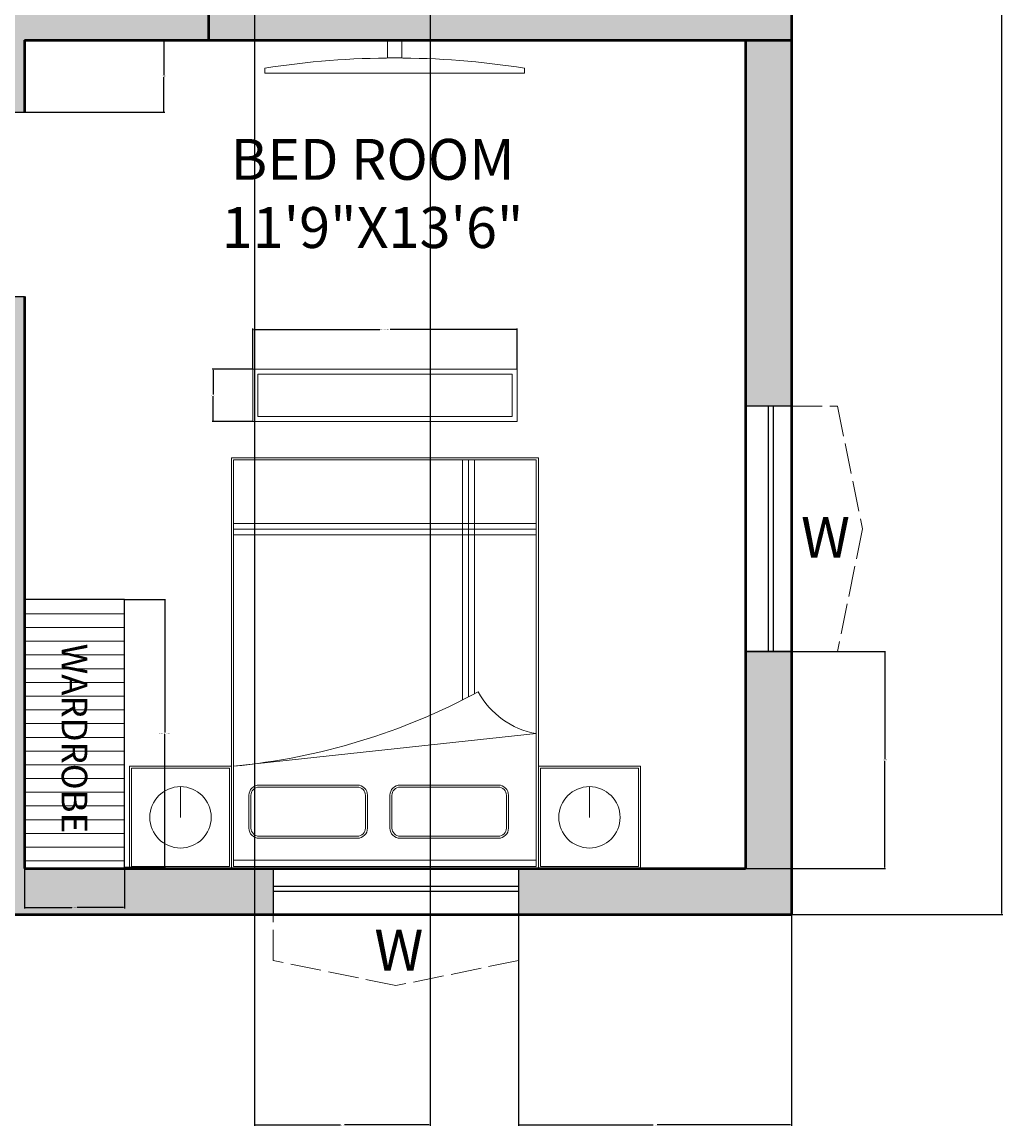
# Model space of a CAD drawing. Units: inches. Extents: x -75 to 416, y -487 to 70.
# Tile 3 of 5: x 224 to 416, y -487 to -271. Entities that reach past the tile are written whole.
import ezdxf

# ---------------------------------------------------------------- set-up
doc = ezdxf.new("R2010")
doc.units = ezdxf.units.IN
doc.header["$MEASUREMENT"] = 0
doc.linetypes.add('ACAD_ISO02W100', pattern=[15, 12, -3])
for name, color, linetype, lineweight in [('A-ANNO-DIMS', 2, 'Continuous', 18), ('A-ANNO-TEXT', 7, 'Continuous', 18), ('A-AREA-IDEN', 7, 'Continuous', 25), ('A-DOOR', 3, 'Continuous', 25), ('A-EQPM', 8, 'Continuous', 18), ('A-FLOR-CASE', 8, 'Continuous', 25), ('A-FLOR-CASE-PATT', 252, 'Continuous', 13), ('A-FURN', 8, 'Continuous', 18), ('A-GLAZ', 4, 'Continuous', 25), ('A-GLAZ-OVHD', 4, 'ACAD_ISO02W100', 13), ('A-WALL', 7, 'Continuous', 50), ('A-WALL-PATT', 252, 'Continuous', 13)]:
    doc.layers.add(name, color=color, linetype=linetype, lineweight=lineweight)
doc.styles.get("Standard").update_dxf_attribs({"font": 'arial.ttf'})
doc.dimstyles.get("Standard").update_dxf_attribs({"dimtxt": 0.18, "dimasz": 0.18, "dimexe": 0.18, "dimexo": 0.0625, "dimgap": 0.09, "dimtad": 0, "dimtih": 1, "dimtoh": 1, "dimdec": 4, "dimzin": 0, "dimdsep": 46, "dimtxsty": 'Standard', "dimcen": 0.09, "dimadec": 0, "dimazin": 0, "dimtfac": 1, "dimtdec": 4, "dimtofl": 0, "dimtmove": 0, "dimatfit": 3, "dimfxl": 1, "dimtolj": 1, "dimtzin": 0, "dimarcsym": 0})

# ---------------------------------------------------------------- blocks, each defined once
blk = doc.blocks.new('A$C0EA4476A')
at = {"linetype": 'ByBlock', "lineweight": -2}
for p, q in [((0, 2.008), (0, 1.508)), ((0.5, 2.008), (0, 2.008)), ((0.01, 1.998), (0.01, 1.518)), ((0.49, 1.998), (0.01, 1.998)), ((0.49, 1.518), (0.49, 1.998)), ((0.5, 2.008), (2, 2.008)), ((0.5, 0), (0.5, 2.008)), ((0.5, 1.508), (0.5, 2.008)), ((0.51, 1.998), (1.99, 1.998)), ((0.51, 0.01), (0.51, 1.998)), ((1.99, 1.998), (1.99, 0.01)), ((2, 2.008), (2, 0)), ((2, 2.008), (2.5, 2.008)), ((2, 1.508), (2, 2.008)), ((2.01, 1.998), (2.49, 1.998)), ((2.01, 1.518), (2.01, 1.998)), ((2.49, 1.998), (2.49, 1.518)), ((2.5, 2.008), (2.5, 1.508)), ((0.51, 1.968), (1.99, 1.968)), ((0.696, 1.8603), (1.176, 1.8603)), ((0.696, 1.8503), (1.176, 1.8503)), ((1.3855, 1.8603), (1.8655, 1.8603)), ((1.3855, 1.8503), (1.8655, 1.8503)), ((0.646, 1.6503), (0.646, 1.8103)), ((0.656, 1.6503), (0.656, 1.8103)), ((1.216, 1.8103), (1.216, 1.6503)), ((1.226, 1.8103), (1.226, 1.6503)), ((1.3355, 1.6503), (1.3355, 1.8103)), ((1.3455, 1.6503), (1.3455, 1.8103)), ((1.9055, 1.8103), (1.9055, 1.6503)), ((1.9155, 1.8103), (1.9155, 1.6503)), ((0.25, 1.758), (0.25, 1.608)), ((2.25, 1.758), (2.25, 1.608)), ((1.176, 1.6103), (0.696, 1.6103)), ((1.176, 1.6003), (0.696, 1.6003)), ((1.8655, 1.6103), (1.3855, 1.6103)), ((1.8655, 1.6003), (1.3855, 1.6003)), ((0.01, 1.518), (0.49, 1.518)), ((2.49, 1.518), (2.01, 1.518)), ((0, 1.508), (0.5, 1.508)), ((1.99, 1.508), (0.51, 1.3488)), ((2.5, 1.508), (2, 1.508)), ((0.8115, 1.1534), (0.8115, 0.01)), ((0.8415, 1.1692), (0.8415, 0.01)), ((0.8715, 1.1845), (0.8715, 0.01)), ((0.51, 0.3775), (1.99, 0.3775)), ((0.51, 0.3495), (1.99, 0.3495)), ((0.51, 0.3216), (1.99, 0.3216)), ((1.99, 0.01), (0.51, 0.01)), ((2, 0), (0.5, 0))]:
    blk.add_line(p, q, dxfattribs=at)
for centre in [(0.25, 1.758), (2.25, 1.758)]:
    blk.add_circle(centre, 0.15, dxfattribs=at)
for centre, radius, start, end in [((0.696, 1.8103), 0.05, 90, 180), ((0.696, 1.8103), 0.04, 90, 180), ((1.176, 1.8103), 0.05, 0, 90), ((1.176, 1.8103), 0.04, 0, 90), ((1.3855, 1.8103), 0.05, 90, 180), ((1.3855, 1.8103), 0.04, 90, 180), ((1.8655, 1.8103), 0.05, 0, 90), ((1.8655, 1.8103), 0.04, 0, 90), ((0.696, 1.6503), 0.05, 180, 270), ((0.696, 1.6503), 0.04, 180, 270), ((1.176, 1.6503), 0.04, 270, 0), ((1.176, 1.6503), 0.05, 270, 0), ((1.3855, 1.6503), 0.05, 180, 270), ((1.3855, 1.6503), 0.04, 180, 270), ((1.8655, 1.6503), 0.05, 270, 0), ((1.8655, 1.6503), 0.04, 270, 0), ((2.2933, -1.6357), 3.1583, 95.5104, 118.3399), ((0.4397, 0.9519), 0.4031, 28.4688, 79.9557)]:
    blk.add_arc(centre, radius, start, end, dxfattribs=at)
blk = doc.blocks.new('A$C1A706E3E')
blk.add_blockref('A$C0EA4476A', (0, 0))
blk = doc.blocks.new('WIN-48IN')
for p, q in [((0, 9), (0, 0)), ((48, 9), (48, 0)), ((48, 5.5), (0, 5.5)), ((48, 4.5), (0, 4.5))]:
    blk.add_line(p, q)
blk = doc.blocks.new('WIN-SHADE-48IN')
at = {"ltscale": 0.5}
for p, q in [((0, 4.91), (0, 13.91)), ((48, 13.91), (48, 4.91)), ((24, 0), (0, 4.91)), ((48, 4.91), (24, 0))]:
    blk.add_line(p, q, dxfattribs=at)
blk = doc.blocks.new('DOOR-36IN')
for p, q in [((0, 9), (0, 0)), ((36, 9), (36, 0)), ((36, 4.5), (0, 4.5))]:
    blk.add_line(p, q)
blk = doc.blocks.new('TV-WALL-MOUNT')
for p, q in [((24, 6.49), (0, 6.49)), ((0, 6.49), (0, 5.49)), ((26.81, 6.49), (24, 6.49)), ((26.81, 6.49), (50.81, 6.49)), ((50.81, 6.49), (50.81, 5.49)), ((24, 3.49), (24, 0)), ((26.81, 3.49), (24, 3.49)), ((26.81, 3.49), (26.81, 0))]:
    blk.add_line(p, q)
blk.add_arc((25.41, 165.85), 162.36, 260.9976, 279.0024)
blk = doc.blocks.new('BENCH-BED-END')
for points in [[(0, 10.24), (51.71, 10.24), (51.71, 0), (0, 0)], [(1, 9.24), (50.71, 9.24), (50.71, 1), (1, 1)]]:
    blk.add_lwpolyline(points, close=True)
blk = doc.blocks.new('WARDROBE-OUTLINE')
for p, q in [((0, 52.38), (0, 0)), ((0, 0), (19.56, 0))]:
    blk.add_line(p, q)
blk = doc.blocks.new('*D24')
at = {"layer": 'A-ANNO-DIMS', "color": 0, "lineweight": -2, "transparency": 16777216}
for p, q in [((269.2, -338.66), (269.2, -330.79)), ((269.38, -330.97), (294.05, -330.97)), ((320.73, -330.97), (296.05, -330.97)), ((320.91, -338.66), (320.91, -330.79))]:
    blk.add_line(p, q, dxfattribs=at)
at = {"layer": 'A-ANNO-DIMS', "color": 0, "transparency": 16777216}
for points in [[(269.38, -330.94), (269.38, -331), (269.2, -330.97)], [(320.73, -330.94), (320.73, -331), (320.91, -330.97)]]:
    blk.add_solid(points, dxfattribs=at)
at = {"layer": 'Defpoints', "color": 0, "transparency": 16777216}
for p in [(320.91, -330.97), (269.2, -338.72), (320.91, -338.72)]:
    blk.add_point(p, dxfattribs=at)
at = {"layer": 'A-ANNO-DIMS', "color": 0, "transparency": 16777216, "insert": (295.05, -330.97), "char_height": 0.18, "attachment_point": 5}
blk.add_mtext('\\A1;BENCH 52 TYP.', dxfattribs=at)
blk = doc.blocks.new('*D25')
at = {"layer": 'A-ANNO-DIMS', "color": 0, "lineweight": -2, "transparency": 16777216}
for p, q in [((269.14, -338.72), (261.26, -338.72)), ((261.44, -338.9), (261.44, -343.66)), ((261.44, -348.78), (261.44, -344.02)), ((269.14, -348.96), (261.26, -348.96))]:
    blk.add_line(p, q, dxfattribs=at)
at = {"layer": 'A-ANNO-DIMS', "color": 0, "transparency": 16777216}
for points in [[(261.41, -338.9), (261.47, -338.9), (261.44, -338.72)], [(261.41, -348.78), (261.47, -348.78), (261.44, -348.96)]]:
    blk.add_solid(points, dxfattribs=at)
at = {"layer": 'Defpoints', "color": 0, "transparency": 16777216}
for p in [(261.44, -338.72), (269.2, -338.72), (269.2, -348.96)]:
    blk.add_point(p, dxfattribs=at)
at = {"layer": 'A-ANNO-DIMS', "color": 0, "transparency": 16777216, "insert": (261.44, -343.84), "char_height": 0.18, "attachment_point": 5}
blk.add_mtext('\\A1;10 TYP.', dxfattribs=at)
blk = doc.blocks.new('*D26')
at = {"layer": 'A-ANNO-DIMS', "color": 0, "lineweight": -2, "transparency": 16777216}
for p, q in [((244.17, -383.76), (252.15, -383.76)), ((251.97, -383.94), (251.97, -409.76)), ((251.97, -435.96), (251.97, -410.13)), ((244.17, -436.14), (252.15, -436.14))]:
    blk.add_line(p, q, dxfattribs=at)
at = {"layer": 'A-ANNO-DIMS', "color": 0, "transparency": 16777216}
for points in [[(251.94, -383.94), (252, -383.94), (251.97, -383.76)], [(251.94, -435.96), (252, -435.96), (251.97, -436.14)]]:
    blk.add_solid(points, dxfattribs=at)
at = {"layer": 'Defpoints', "color": 0, "transparency": 16777216}
for p in [(244.11, -383.76), (244.11, -436.14), (251.97, -436.14)]:
    blk.add_point(p, dxfattribs=at)
at = {"layer": 'A-ANNO-DIMS', "color": 0, "transparency": 16777216, "insert": (251.97, -409.95), "char_height": 0.18, "attachment_point": 5}
blk.add_mtext('\\A1;WARDROBE 52 TYP.', dxfattribs=at)
blk = doc.blocks.new('*D27')
at = {"layer": 'A-ANNO-DIMS', "color": 0, "lineweight": -2, "transparency": 16777216}
for p, q in [((224.55, -436.2), (224.55, -444.17)), ((244.11, -436.2), (244.11, -444.17)), ((224.73, -443.99), (233.8, -443.99)), ((243.93, -443.99), (234.86, -443.99))]:
    blk.add_line(p, q, dxfattribs=at)
at = {"layer": 'A-ANNO-DIMS', "color": 0, "transparency": 16777216}
for points in [[(224.73, -443.96), (224.73, -444.02), (224.55, -443.99)], [(243.93, -443.96), (243.93, -444.02), (244.11, -443.99)]]:
    blk.add_solid(points, dxfattribs=at)
at = {"layer": 'Defpoints', "color": 0, "transparency": 16777216}
for p in [(224.55, -436.14), (244.11, -436.14), (224.55, -443.99)]:
    blk.add_point(p, dxfattribs=at)
at = {"layer": 'A-ANNO-DIMS', "color": 0, "transparency": 16777216, "insert": (234.33, -443.99), "char_height": 0.18, "attachment_point": 5}
blk.add_mtext('\\A1;20 TYP.', dxfattribs=at)
blk = doc.blocks.new('*D35')
at = {"layer": 'A-ANNO-DIMS', "color": 0, "lineweight": -2, "transparency": 16777216}
for p, q in [((374.615553, 28.625508), (415.902741, 28.625508)), ((415.722741, 28.445508), (415.722741, -208.194492)), ((415.722741, -445.194492), (415.722741, -208.554492)), ((374.615553, -445.374492), (415.902741, -445.374492))]:
    blk.add_line(p, q, dxfattribs=at)
at = {"layer": 'A-ANNO-DIMS', "color": 0, "transparency": 16777216}
for points in [[(415.692741, 28.445508), (415.752741, 28.445508), (415.722741, 28.625508)], [(415.692741, -445.194492), (415.752741, -445.194492), (415.722741, -445.374492)]]:
    blk.add_solid(points, dxfattribs=at)
at = {"layer": 'Defpoints', "color": 0, "transparency": 16777216}
for p in [(374.553053, 28.625508), (374.553053, -445.374492), (415.722741, -445.374492)]:
    blk.add_point(p, dxfattribs=at)
at = {"layer": 'A-ANNO-DIMS', "color": 0, "transparency": 16777216, "insert": (415.722741, -208.374492), "char_height": 0.18, "attachment_point": 5}
blk.add_mtext('\\A1;474', dxfattribs=at)
blk = doc.blocks.new('*D42')
at = {"layer": 'A-ANNO-DIMS', "color": 0, "lineweight": -2, "transparency": 16777216}
for p, q in [((365.62, -393.93), (392.99, -393.93)), ((392.81, -394.11), (392.81, -414.97)), ((392.81, -436.19), (392.81, -415.33)), ((365.62, -436.37), (392.99, -436.37))]:
    blk.add_line(p, q, dxfattribs=at)
at = {"layer": 'A-ANNO-DIMS', "color": 0, "transparency": 16777216}
for points in [[(392.78, -394.11), (392.84, -394.11), (392.81, -393.93)], [(392.78, -436.19), (392.84, -436.19), (392.81, -436.37)]]:
    blk.add_solid(points, dxfattribs=at)
at = {"layer": 'Defpoints', "color": 0, "transparency": 16777216}
for p in [(365.55, -393.93), (365.55, -436.37), (392.81, -436.37)]:
    blk.add_point(p, dxfattribs=at)
at = {"layer": 'A-ANNO-DIMS', "color": 0, "transparency": 16777216, "insert": (392.81, -415.15), "char_height": 0.18, "attachment_point": 5}
blk.add_mtext('\\A1;42.444', dxfattribs=at)
blk = doc.blocks.new('*D51')
at = {"layer": 'A-ANNO-DIMS', "color": 0, "lineweight": -2, "transparency": 16777216}
for p, q in [((321.2, -445.44), (321.2, -486.72)), ((374.55, -445.44), (374.55, -486.72)), ((321.38, -486.54), (347.48, -486.54)), ((374.37, -486.54), (348.27, -486.54))]:
    blk.add_line(p, q, dxfattribs=at)
at = {"layer": 'A-ANNO-DIMS', "color": 0, "transparency": 16777216}
for points in [[(321.38, -486.51), (321.38, -486.57), (321.2, -486.54)], [(374.37, -486.51), (374.37, -486.57), (374.55, -486.54)]]:
    blk.add_solid(points, dxfattribs=at)
at = {"layer": 'Defpoints', "color": 0, "transparency": 16777216}
for p in [(321.2, -445.37), (374.55, -445.37), (321.2, -486.54)]:
    blk.add_point(p, dxfattribs=at)
at = {"layer": 'A-ANNO-DIMS', "color": 0, "transparency": 16777216, "insert": (347.88, -486.54), "char_height": 0.18, "attachment_point": 5}
blk.add_mtext('\\A1;53.35', dxfattribs=at)
blk = doc.blocks.new('*D56')
at = {"layer": 'A-ANNO-DIMS', "color": 0, "lineweight": -2, "transparency": 16777216}
for p, q in [((224.62, -274.37), (251.99, -274.37)), ((251.81, -274.55), (251.81, -281.25)), ((251.81, -288.31), (251.81, -281.61)), ((224.62, -288.49), (251.99, -288.49))]:
    blk.add_line(p, q, dxfattribs=at)
at = {"layer": 'A-ANNO-DIMS', "color": 0, "transparency": 16777216}
for points in [[(251.78, -274.55), (251.84, -274.55), (251.81, -274.37)], [(251.78, -288.31), (251.84, -288.31), (251.81, -288.49)]]:
    blk.add_solid(points, dxfattribs=at)
at = {"layer": 'Defpoints', "color": 0, "transparency": 16777216}
for p in [(224.55, -274.37), (224.55, -288.49), (251.81, -288.49)]:
    blk.add_point(p, dxfattribs=at)
at = {"layer": 'A-ANNO-DIMS', "color": 0, "transparency": 16777216, "insert": (251.81, -281.43), "char_height": 0.18, "attachment_point": 5}
blk.add_mtext('\\A1;14.116', dxfattribs=at)
blk = doc.blocks.new('*D71')
at = {"layer": 'A-ANNO-DIMS', "color": 0, "lineweight": -2, "transparency": 16777216}
for p, q in [((303.87, -261.95), (303.87, -486.72)), ((269.55, -265.44), (269.55, -486.72)), ((269.73, -486.54), (286.32, -486.54)), ((303.69, -486.54), (287.11, -486.54))]:
    blk.add_line(p, q, dxfattribs=at)
at = {"layer": 'A-ANNO-DIMS', "color": 0, "transparency": 16777216}
for points in [[(269.73, -486.51), (269.73, -486.57), (269.55, -486.54)], [(303.69, -486.51), (303.69, -486.57), (303.87, -486.54)]]:
    blk.add_solid(points, dxfattribs=at)
at = {"layer": 'Defpoints', "color": 0, "transparency": 16777216}
for p in [(303.87, -261.88), (269.55, -265.37), (303.87, -486.54)]:
    blk.add_point(p, dxfattribs=at)
at = {"layer": 'A-ANNO-DIMS', "color": 0, "transparency": 16777216, "insert": (286.71, -486.54), "char_height": 0.18, "attachment_point": 5}
blk.add_mtext('\\A1;34.32', dxfattribs=at)

msp = doc.modelspace()

# ---------------------------------------------------------------- hatches: boundary and pattern name
at = {"layer": 'A-FLOR-CASE-PATT'}
h = msp.add_hatch(dxfattribs=at)
h.set_pattern_fill('ANSI31', color=256, scale=21.476, angle=-45, style=0)
h.paths.add_polyline_path([(224.5531, -436.1079), (244.1093, -436.1079), (244.1093, -385.1024), (224.5531, -385.1024)])
at = {"layer": 'A-WALL-PATT'}
h = msp.add_hatch(color=256, dxfattribs=at)
h.dxf.hatch_style = 1
h.paths.add_polyline_path([(84.8603, 28.6255), (3.5531, 28.6255), (3.5531, -23.8141), (12.5531, -23.8141), (12.5531, 19.6255), (84.8603, 19.6255)])
h.paths.add_polyline_path([(263.7442, 28.6255), (132.8603, 28.6255), (132.8603, 19.6255), (146.5531, 19.6255), (180.5531, 19.6255), (180.5531, -124.3745), (180.5531, -133.3745), (200.467, -133.3745), (200.467, -124.3745), (189.5531, -124.3745), (189.5531, 19.6255), (263.7442, 19.6255)])
h.paths.add_polyline_path([(374.5531, 28.6255), (311.7442, 28.6255), (311.7442, 19.6255), (327.5531, 19.6255), (365.5531, 19.6255), (365.5531, -37.0191), (374.5531, -37.0191)])
h.paths.add_polyline_path([(144.5531, -124.3745), (12.5531, -124.3745), (12.5531, -71.8141), (3.5531, -71.8141), (3.5531, -148.6403), (12.5531, -148.6403), (12.5531, -133.3745), (144.5531, -133.3745)])
h.paths.add_polyline_path([(117.5531, -133.3745), (108.5531, -133.3745), (108.5531, -161.7866), (117.5531, -161.7866)])
h.paths.add_polyline_path([(374.5531, -85.0191), (365.5531, -85.0191), (365.5531, -124.3745), (236.467, -124.3745), (236.467, -133.3745), (374.5531, -133.3745)])
h.paths.add_polyline_path([(374.5531, -133.3745), (365.5531, -133.3745), (365.5531, -183.1692), (374.5531, -183.1692)])
h.paths.add_polyline_path([(374.5531, -231.1692), (365.5531, -231.1692), (365.5531, -265.3745), (260.5531, -265.3745), (260.5531, -274.3745), (374.5531, -274.3745)])
h.paths.add_polyline_path([(260.5531, -265.3745), (215.5531, -265.3745), (215.5531, -288.4908), (224.5531, -288.4908), (224.5531, -274.3745), (260.5531, -274.3745)])
h.paths.add_polyline_path([(374.5531, -274.3745), (365.5531, -274.3745), (365.5531, -345.9302), (374.5531, -345.9302)])
h.paths.add_polyline_path([(374.5531, -393.9302), (365.5531, -393.9302), (365.5531, -436.3745), (321.1982, -436.3745), (321.1982, -445.3745), (374.5531, -445.3745)])
h.paths.add_polyline_path([(224.5531, -324.4908), (215.5531, -324.4908), (215.5531, -445.3745), (273.1982, -445.3745), (273.1982, -436.3745), (265.0531, -436.3745), (245.0531, -436.3745), (224.5531, -436.3745)])
h.paths.add_polyline_path([(12.5531, -183.233), (3.5531, -183.233), (3.5531, -214.3745), (117.5531, -214.3745), (117.5531, -197.7866), (108.5531, -197.7866), (108.5531, -205.3745), (12.5531, -205.3745)])
h.paths.add_polyline_path([(12.5531, -214.3745), (3.5531, -214.3745), (3.5531, -290.2477), (12.5531, -290.2477)])
h.paths.add_polyline_path([(75.0426, -381.3745), (12.5531, -381.3745), (12.5531, -350.2477), (3.5531, -350.2477), (3.5531, -390.3745), (75.0426, -390.3745)])
h.paths.add_polyline_path([(154.4537, -381.3745), (123.0426, -381.3745), (123.0426, -390.3745), (154.4537, -390.3745)])
h.paths.add_polyline_path([(215.5531, -381.3745), (202.4537, -381.3745), (202.4537, -390.3745), (215.5531, -390.3745)])

# ---------------------------------------------------------------- linework, layer by layer
at = {"layer": 'A-WALL'}
for p, q in [((374.5531, 28.6255), (374.5531, -445.3745)), ((260.5531, -225.367), (260.5531, -274.3745)), ((224.5531, -274.3745), (374.5531, -274.3745)), ((224.5531, -274.3745), (224.5531, -288.4908)), ((365.5531, -274.3745), (365.5531, -436.3745)), ((224.5531, -324.4908), (224.5531, -436.3745)), ((224.5531, -436.3745), (365.5531, -436.3745)), ((215.5531, -445.3745), (374.5531, -445.3745))]:
    msp.add_line(p, q, dxfattribs=at)

# ---------------------------------------------------------------- block references
at = {"layer": 'A-DOOR', "rotation": 89.99999999999999}
msp.add_blockref('DOOR-36IN', (224.5526, -324.4909), dxfattribs=at)
at = {"layer": 'A-EQPM', "rotation": 180}
msp.add_blockref('TV-WALL-MOUNT', (322.3515, -274.375), dxfattribs=at)
at = {"layer": 'A-FLOR-CASE', "rotation": 180}
msp.add_blockref('WARDROBE-OUTLINE', (244.1091, -383.7602), dxfattribs=at)
at = {"layer": 'A-FURN'}
msp.add_blockref('BENCH-BED-END', (269.1997, -348.9615), dxfattribs=at)
at = {"layer": 'A-FURN', "xscale": 40.00000000000001, "yscale": 40.00000000000001, "zscale": 40.00000000000001, "rotation": 180}
msp.add_blockref('A$C1A706E3E', (345.053, -356.0545), dxfattribs=at)
at = {"layer": 'A-GLAZ', "rotation": 270.0000000000004}
msp.add_blockref('WIN-48IN', (365.5535, -345.9306), dxfattribs=at)
at = {"layer": 'A-GLAZ'}
msp.add_blockref('WIN-48IN', (273.1987, -445.374), dxfattribs=at)
at = {"layer": 'A-GLAZ-OVHD', "rotation": 89.99999999999984}
msp.add_blockref('WIN-SHADE-48IN', (388.4626, -393.9304), dxfattribs=at)
at = {"layer": 'A-GLAZ-OVHD'}
msp.add_blockref('WIN-SHADE-48IN', (273.198, -459.284), dxfattribs=at)

# ---------------------------------------------------------------- texts
at = {"layer": 'A-ANNO-TEXT', "char_height": 8, "attachment_point": 1}
for insert in [(373.6583, -367.6192), (290.2003, -448.3452)]:
    msp.add_mtext_dynamic_manual_height_columns('\\pxqc;W', width=15.130285, gutter_width=1, heights=[0], dxfattribs=dict(at, insert=insert))
at = {"layer": 'A-ANNO-TEXT', "insert": (236.8138, -338.7495), "char_height": 5, "attachment_point": 1, "rotation": 270}
msp.add_mtext_dynamic_manual_height_columns('\\pxqc;WARDROBE', width=144.357858, gutter_width=1, heights=[0], dxfattribs=at)
at = {"layer": 'A-AREA-IDEN', "insert": (220.4438, -293.6895), "char_height": 8, "attachment_point": 1}
msp.add_mtext_dynamic_manual_height_columns('\\pxqc;BED ROOM\\P11\'9"X13\'6"', width=144.357858, gutter_width=1, heights=[0], dxfattribs=at)

# ---------------------------------------------------------------- dimensions: what is measured, and where the dimension line sits
at = {"layer": 'A-ANNO-DIMS'}
for base, p1, p2, angle, override, picture, middle in [((415.7227, -445.3745), (374.5531, 28.6255), (374.5531, -445.3745), 90, {"dimdec": 0, "dimlfac": 1, "dimrnd": 0, "dimzin": 0, "dimdsep": 46, "dimlunit": 2}, '*D35', (415.7227, -208.3745)), ((251.8131, -288.4908), (224.5531, -274.3745), (224.5531, -288.4908), 270, {"dimdec": 3, "dimlfac": 1, "dimrnd": 0, "dimzin": 0, "dimdsep": 46, "dimlunit": 2}, '*D56', (251.8131, -281.4327)), ((392.8131, -436.3745), (365.5531, -393.9302), (365.5531, -436.3745), 270, {"dimdec": 3, "dimlfac": 1, "dimrnd": 0, "dimzin": 0, "dimdsep": 46, "dimlunit": 2}, '*D42', (392.8131, -415.1523))]:
    dim = msp.add_linear_dim(base=base, p1=p1, p2=p2, angle=angle, dimstyle='Standard', override=override, dxfattribs=at)
    dim.commit()
    dim.dimension.update_dxf_attribs({"geometry": picture, "text_midpoint": middle})
for base, p1, p2, picture, middle in [((303.8724, -486.5442), (269.5531, -265.3745), (303.8724, -261.883), '*D71', (286.7127, -486.5442)), ((321.1982, -486.5442), (374.5531, -445.3745), (321.1982, -445.3745), '*D51', (347.8756, -486.5442))]:
    dim = msp.add_linear_dim(base=base, p1=p1, p2=p2, dimstyle='Standard', override={"dimdec": 2, "dimlfac": 1, "dimrnd": 0, "dimzin": 0, "dimdsep": 46, "dimlunit": 2}, dxfattribs=at)
    dim.commit()
    dim.dimension.update_dxf_attribs({"geometry": picture, "text_midpoint": middle})
dim = msp.add_linear_dim(base=(320.9065, -330.9676), p1=(269.1996, -338.7236), p2=(320.9065, -338.7236), text='BENCH <> TYP.', dimstyle='Standard', override={"dimdec": 0, "dimlfac": 1, "dimrnd": 0, "dimzin": 0, "dimdsep": 46, "dimlunit": 2}, dxfattribs=at)
dim.commit()
dim.dimension.update_dxf_attribs({"geometry": '*D24', "text_midpoint": (295.0531, -330.9676)})
for base, p1, p2, angle, text, picture, middle in [((261.4436, -338.7236), (269.1996, -348.9618), (269.1996, -338.7236), 90, '<> TYP.', '*D25', (261.4436, -343.8427)), ((251.9656, -436.1357), (244.1093, -383.7601), (244.1093, -436.1357), 270, 'WARDROBE <> TYP.', '*D26', (251.9656, -409.9479)), ((224.5531, -443.9921), (244.1093, -436.1357), (224.5531, -436.1357), 180, '<> TYP.', '*D27', (234.3312, -443.9921))]:
    dim = msp.add_linear_dim(base=base, p1=p1, p2=p2, angle=angle, text=text, dimstyle='Standard', override={"dimdec": 0, "dimlfac": 1, "dimrnd": 0, "dimzin": 0, "dimdsep": 46, "dimlunit": 2}, dxfattribs=at)
    dim.commit()
    dim.dimension.update_dxf_attribs({"geometry": picture, "text_midpoint": middle})

doc.saveas('drawing.dxf')
